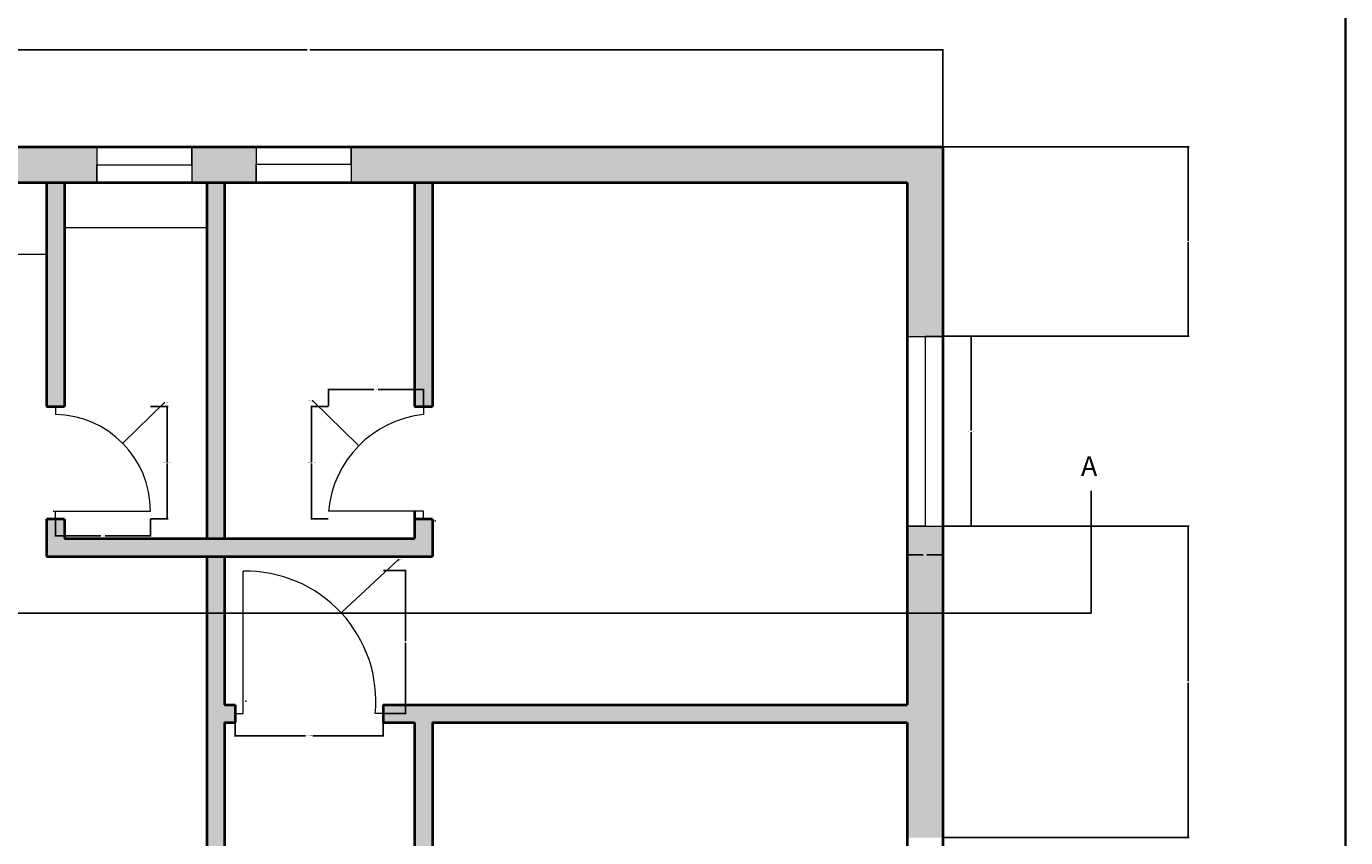
# Model space of a CAD drawing. Units: inches. Extents: x 1441 to 2460, y 1648 to 2683.
# Tile 33 of 35: x 2127 to 2460, y 2124 to 2329. Entities that reach past the tile are written whole.
import ezdxf

# ---------------------------------------------------------------- set-up
doc = ezdxf.new("R2010")
doc.units = ezdxf.units.IN
for name, color, linetype, lineweight in [('A-ANNO-DIMS', 2, 'Continuous', 18), ('A-ANNO-SYMB', 5, 'Continuous', 25), ('A-ANNO-TTLB', 7, 'Continuous', 35), ('A-DOOR', 3, 'Continuous', 20), ('A-FLOR-CASE', 9, 'Continuous', 20), ('A-GLAZ', 4, 'Continuous', 18), ('A-WALL', 7, 'Continuous', 40)]:
    doc.layers.add(name, color=color, linetype=linetype, lineweight=lineweight)
doc.layers.add('A-WALL-PATT', color=251, linetype='Continuous', lineweight=13, true_color=0x636466)
doc.styles.get("Standard").update_dxf_attribs({"font": 'arial.ttf'})
doc.dimstyles.get("Standard").update_dxf_attribs({"dimtxt": 0.18, "dimasz": 0.18, "dimexe": 0.18, "dimexo": 0.0625, "dimgap": 0.09, "dimtad": 0, "dimtih": 1, "dimtoh": 1, "dimdec": 4, "dimzin": 0, "dimdsep": 46, "dimtxsty": 'Standard', "dimcen": 0.09, "dimadec": 0, "dimazin": 0, "dimtfac": 1, "dimtdec": 4, "dimtofl": 0, "dimtmove": 0, "dimatfit": 3, "dimfxl": 1, "dimtolj": 1, "dimtzin": 0, "dimarcsym": 0})

# ---------------------------------------------------------------- blocks, each defined once
blk = doc.blocks.new('DOOR-BED1-36')
for p, q in [((2, 0), (2, 36)), ((0, 0), (2, 0)), ((37.39, 0), (35.39, 0))]:
    blk.add_line(p, q)
blk.add_arc((2.69, 3.15), 32.85, 354.488, 91.1985)
blk = doc.blocks.new('DOOR-WC-NORTH-24')
for p, q in [((24, 28.42), (24, 26.42)), ((24, 2), (0, 2)), ((24, 0), (24, 2))]:
    blk.add_line(p, q)
blk.add_arc((26.92, -0.45), 27.04, 96.2058, 174.7965)
blk = doc.blocks.new('DOOR-STORE-24')
for p, q in [((0, 28.42), (0, 26.42)), ((0, 0), (0, 2)), ((0, 2), (24, 2))]:
    blk.add_line(p, q)
blk.add_arc((-0.43, 2), 24.43, 0, 88.9938)
blk = doc.blocks.new('WIN-48-SASH')
for p, q in [((9, 48), (4.5, 48)), ((4.5, 48), (4.5, 0)), ((4.5, 0), (0, 0))]:
    blk.add_line(p, q)
blk = doc.blocks.new('*D42')
at = {"layer": 'A-ANNO-DIMS', "color": 0, "lineweight": -2, "transparency": 16777216}
for p, q in [((2179.58, 2155.38), (2179.58, 2149.66)), ((2216.96, 2155.38), (2216.96, 2149.66)), ((2179.76, 2149.84), (2197.34, 2149.84)), ((2216.78, 2149.84), (2199.2, 2149.84))]:
    blk.add_line(p, q, dxfattribs=at)
at = {"layer": 'A-ANNO-DIMS', "color": 0, "transparency": 16777216}
for points in [[(2179.76, 2149.87), (2179.76, 2149.81), (2179.58, 2149.84)], [(2216.78, 2149.87), (2216.78, 2149.81), (2216.96, 2149.84)]]:
    blk.add_solid(points, dxfattribs=at)
at = {"layer": 'Defpoints', "color": 0, "transparency": 16777216}
for p in [(2179.58, 2155.45), (2216.96, 2155.45), (2216.96, 2149.84)]:
    blk.add_point(p, dxfattribs=at)
at = {"layer": 'A-ANNO-DIMS', "color": 0, "transparency": 16777216, "insert": (2198.27, 2149.84), "char_height": 0.18, "attachment_point": 5}
blk.add_mtext('\\A1;B1 DR 37 TYP.', dxfattribs=at)
blk = doc.blocks.new('*D43')
at = {"layer": 'A-ANNO-DIMS', "color": 0, "lineweight": -2, "transparency": 16777216}
for p, q in [((2217.03, 2191.64), (2222.75, 2191.64)), ((2222.57, 2191.46), (2222.57, 2173.73)), ((2222.57, 2155.63), (2222.57, 2173.36)), ((2217.03, 2155.45), (2222.75, 2155.45))]:
    blk.add_line(p, q, dxfattribs=at)
at = {"layer": 'A-ANNO-DIMS', "color": 0, "transparency": 16777216}
for points in [[(2222.54, 2191.46), (2222.6, 2191.46), (2222.57, 2191.64)], [(2222.54, 2155.63), (2222.6, 2155.63), (2222.57, 2155.45)]]:
    blk.add_solid(points, dxfattribs=at)
at = {"layer": 'Defpoints', "color": 0, "transparency": 16777216}
for p in [(2216.96, 2191.64), (2222.57, 2191.64), (2216.96, 2155.45)]:
    blk.add_point(p, dxfattribs=at)
at = {"layer": 'A-ANNO-DIMS', "color": 0, "transparency": 16777216, "insert": (2222.57, 2173.54), "char_height": 0.18, "attachment_point": 5}
blk.add_mtext('\\A1;36 TYP.', dxfattribs=at)
blk = doc.blocks.new('*D44')
at = {"layer": 'A-ANNO-DIMS', "color": 0, "lineweight": -2, "transparency": 16777216}
for p, q in [((2203.09, 2233.06), (2198.71, 2233.06)), ((2198.89, 2232.88), (2198.89, 2219.03)), ((2198.89, 2204.82), (2198.89, 2218.67)), ((2203.09, 2204.64), (2198.71, 2204.64))]:
    blk.add_line(p, q, dxfattribs=at)
at = {"layer": 'A-ANNO-DIMS', "color": 0, "transparency": 16777216}
for points in [[(2198.86, 2232.88), (2198.92, 2232.88), (2198.89, 2233.06)], [(2198.86, 2204.82), (2198.92, 2204.82), (2198.89, 2204.64)]]:
    blk.add_solid(points, dxfattribs=at)
at = {"layer": 'Defpoints', "color": 0, "transparency": 16777216}
for p in [(2198.89, 2233.06), (2203.15, 2233.06), (2203.15, 2204.64)]:
    blk.add_point(p, dxfattribs=at)
at = {"layer": 'A-ANNO-DIMS', "color": 0, "transparency": 16777216, "insert": (2198.89, 2218.85), "char_height": 0.18, "attachment_point": 5}
blk.add_mtext('\\A1;WC DOOR 28 TYP.', dxfattribs=at)
blk = doc.blocks.new('*D45')
at = {"layer": 'A-ANNO-DIMS', "color": 0, "lineweight": -2, "transparency": 16777216}
for p, q in [((2203.15, 2233.12), (2203.15, 2237.51)), ((2203.33, 2237.33), (2214.62, 2237.33)), ((2226.97, 2237.33), (2215.68, 2237.33)), ((2227.15, 2233.12), (2227.15, 2237.51))]:
    blk.add_line(p, q, dxfattribs=at)
at = {"layer": 'A-ANNO-DIMS', "color": 0, "transparency": 16777216}
for points in [[(2203.33, 2237.36), (2203.33, 2237.3), (2203.15, 2237.33)], [(2226.97, 2237.36), (2226.97, 2237.3), (2227.15, 2237.33)]]:
    blk.add_solid(points, dxfattribs=at)
at = {"layer": 'Defpoints', "color": 0, "transparency": 16777216}
for p in [(2227.15, 2237.33), (2203.15, 2233.06), (2227.15, 2233.06)]:
    blk.add_point(p, dxfattribs=at)
at = {"layer": 'A-ANNO-DIMS', "color": 0, "transparency": 16777216, "insert": (2215.15, 2237.33), "char_height": 0.18, "attachment_point": 5}
blk.add_mtext('\\A1;24 TYP.', dxfattribs=at)
blk = doc.blocks.new('*D46')
at = {"layer": 'A-ANNO-DIMS', "color": 0, "lineweight": -2, "transparency": 16777216}
for p, q in [((2158.21, 2233.06), (2162.6, 2233.06)), ((2162.42, 2232.88), (2162.42, 2219.03)), ((2162.42, 2204.82), (2162.42, 2218.67)), ((2158.21, 2204.64), (2162.6, 2204.64))]:
    blk.add_line(p, q, dxfattribs=at)
at = {"layer": 'A-ANNO-DIMS', "color": 0, "transparency": 16777216}
for points in [[(2162.39, 2232.88), (2162.45, 2232.88), (2162.42, 2233.06)], [(2162.39, 2204.82), (2162.45, 2204.82), (2162.42, 2204.64)]]:
    blk.add_solid(points, dxfattribs=at)
at = {"layer": 'Defpoints', "color": 0, "transparency": 16777216}
for p in [(2158.15, 2233.06), (2162.42, 2233.06), (2158.15, 2204.64)]:
    blk.add_point(p, dxfattribs=at)
at = {"layer": 'A-ANNO-DIMS', "color": 0, "transparency": 16777216, "insert": (2162.42, 2218.85), "char_height": 0.18, "attachment_point": 5}
blk.add_mtext('\\A1;STORE DOOR 28 TYP.', dxfattribs=at)
blk = doc.blocks.new('*D47')
at = {"layer": 'A-ANNO-DIMS', "color": 0, "lineweight": -2, "transparency": 16777216}
for p, q in [((2134.15, 2204.57), (2134.15, 2200.19)), ((2158.15, 2204.57), (2158.15, 2200.19)), ((2134.33, 2200.37), (2145.62, 2200.37)), ((2157.97, 2200.37), (2146.68, 2200.37))]:
    blk.add_line(p, q, dxfattribs=at)
at = {"layer": 'A-ANNO-DIMS', "color": 0, "transparency": 16777216}
for points in [[(2134.33, 2200.4), (2134.33, 2200.34), (2134.15, 2200.37)], [(2157.97, 2200.4), (2157.97, 2200.34), (2158.15, 2200.37)]]:
    blk.add_solid(points, dxfattribs=at)
at = {"layer": 'Defpoints', "color": 0, "transparency": 16777216}
for p in [(2134.15, 2204.64), (2158.15, 2204.64), (2158.15, 2200.37)]:
    blk.add_point(p, dxfattribs=at)
at = {"layer": 'A-ANNO-DIMS', "color": 0, "transparency": 16777216, "insert": (2146.15, 2200.37), "char_height": 0.18, "attachment_point": 5}
blk.add_mtext('\\A1;24 TYP.', dxfattribs=at)
blk = doc.blocks.new('*D58')
at = {"layer": 'A-ANNO-DIMS', "color": 0, "lineweight": -2, "transparency": 16777216}
for p, q in [((2358.46, 2250.81), (2365.78, 2250.81)), ((2365.6, 2250.63), (2365.6, 2226.99)), ((2365.6, 2202.99), (2365.6, 2226.62)), ((2358.46, 2202.81), (2365.78, 2202.81))]:
    blk.add_line(p, q, dxfattribs=at)
at = {"layer": 'A-ANNO-DIMS', "color": 0, "transparency": 16777216}
for points in [[(2365.57, 2250.63), (2365.63, 2250.63), (2365.6, 2250.81)], [(2365.57, 2202.99), (2365.63, 2202.99), (2365.6, 2202.81)]]:
    blk.add_solid(points, dxfattribs=at)
at = {"layer": 'Defpoints', "color": 0, "transparency": 16777216}
for p in [(2358.4, 2250.81), (2365.6, 2250.81), (2358.4, 2202.81)]:
    blk.add_point(p, dxfattribs=at)
at = {"layer": 'A-ANNO-DIMS', "color": 0, "transparency": 16777216, "insert": (2365.6, 2226.81), "char_height": 0.18, "attachment_point": 5}
blk.add_mtext('\\A1;SASH 48 TYP.', dxfattribs=at)
blk = doc.blocks.new('*D59')
at = {"layer": 'A-ANNO-DIMS', "color": 0, "lineweight": -2, "transparency": 16777216}
for p, q in [((2349.4, 2202.74), (2349.4, 2195.43)), ((2358.4, 2202.74), (2358.4, 2195.43)), ((2349.58, 2195.61), (2353.44, 2195.61)), ((2358.22, 2195.61), (2354.36, 2195.61))]:
    blk.add_line(p, q, dxfattribs=at)
at = {"layer": 'A-ANNO-DIMS', "color": 0, "transparency": 16777216}
for points in [[(2349.58, 2195.64), (2349.58, 2195.58), (2349.4, 2195.61)], [(2358.22, 2195.64), (2358.22, 2195.58), (2358.4, 2195.61)]]:
    blk.add_solid(points, dxfattribs=at)
at = {"layer": 'Defpoints', "color": 0, "transparency": 16777216}
for p in [(2349.4, 2202.81), (2358.4, 2202.81), (2358.4, 2195.61)]:
    blk.add_point(p, dxfattribs=at)
at = {"layer": 'A-ANNO-DIMS', "color": 0, "transparency": 16777216, "insert": (2353.9, 2195.61), "char_height": 0.18, "attachment_point": 5}
blk.add_mtext('\\A1;9 TYP.', dxfattribs=at)
blk = doc.blocks.new('*D80')
at = {"layer": 'A-ANNO-DIMS', "color": 0, "lineweight": -2, "transparency": 16777216}
for p, q in [((2037.9, 2298.76), (2037.9, 2323.43)), ((2038.08, 2323.25), (2197.76, 2323.25)), ((2358.22, 2323.25), (2198.55, 2323.25)), ((2358.4, 2298.76), (2358.4, 2323.43))]:
    blk.add_line(p, q, dxfattribs=at)
at = {"layer": 'A-ANNO-DIMS', "color": 0, "transparency": 16777216}
for points in [[(2038.08, 2323.28), (2038.08, 2323.22), (2037.9, 2323.25)], [(2358.22, 2323.28), (2358.22, 2323.22), (2358.4, 2323.25)]]:
    blk.add_solid(points, dxfattribs=at)
at = {"layer": 'Defpoints', "color": 0, "transparency": 16777216}
for p in [(2358.4, 2323.25), (2037.9, 2298.7), (2358.4, 2298.7)]:
    blk.add_point(p, dxfattribs=at)
at = {"layer": 'A-ANNO-DIMS', "color": 0, "transparency": 16777216, "insert": (2198.15, 2323.25), "char_height": 0.18, "attachment_point": 5}
blk.add_mtext('\\A1;320.5', dxfattribs=at)
blk = doc.blocks.new('*D81')
at = {"layer": 'A-ANNO-DIMS', "color": 0, "lineweight": -2, "transparency": 16777216}
for p, q in [((2037.84, 2298.7), (1976.42, 2298.7)), ((1976.6, 2298.52), (1976.6, 2055.94)), ((1976.6, 1813), (1976.6, 2055.57)), ((2154.24, 1812.82), (1976.42, 1812.82))]:
    blk.add_line(p, q, dxfattribs=at)
at = {"layer": 'A-ANNO-DIMS', "color": 0, "transparency": 16777216}
for points in [[(1976.57, 2298.52), (1976.63, 2298.52), (1976.6, 2298.7)], [(1976.57, 1813), (1976.63, 1813), (1976.6, 1812.82)]]:
    blk.add_solid(points, dxfattribs=at)
at = {"layer": 'Defpoints', "color": 0, "transparency": 16777216}
for p in [(1976.6, 2298.7), (2037.9, 2298.7), (2154.3, 1812.82)]:
    blk.add_point(p, dxfattribs=at)
at = {"layer": 'A-ANNO-DIMS', "color": 0, "transparency": 16777216, "insert": (1976.6, 2055.76), "char_height": 0.18, "attachment_point": 5}
blk.add_mtext('\\A1;485.9', dxfattribs=at)
blk = doc.blocks.new('*D88')
at = {"layer": 'A-ANNO-DIMS', "color": 0, "lineweight": -2, "transparency": 16777216}
for p, q in [((2358.46, 2202.81), (2420.62, 2202.81)), ((2420.44, 2202.63), (2420.44, 2163.64)), ((2420.44, 2124.29), (2420.44, 2163.27)), ((2358.46, 2124.11), (2420.62, 2124.11))]:
    blk.add_line(p, q, dxfattribs=at)
at = {"layer": 'A-ANNO-DIMS', "color": 0, "transparency": 16777216}
for points in [[(2420.41, 2202.63), (2420.47, 2202.63), (2420.44, 2202.81)], [(2420.41, 2124.29), (2420.47, 2124.29), (2420.44, 2124.11)]]:
    blk.add_solid(points, dxfattribs=at)
at = {"layer": 'Defpoints', "color": 0, "transparency": 16777216}
for p in [(2358.4, 2202.81), (2420.44, 2202.81), (2358.4, 2124.11)]:
    blk.add_point(p, dxfattribs=at)
at = {"layer": 'A-ANNO-DIMS', "color": 0, "transparency": 16777216, "insert": (2420.44, 2163.46), "char_height": 0.18, "attachment_point": 5}
blk.add_mtext('\\A1;78.7', dxfattribs=at)
blk = doc.blocks.new('*D89')
at = {"layer": 'A-ANNO-DIMS', "color": 0, "lineweight": -2, "transparency": 16777216}
for p, q in [((2358.46, 2298.7), (2420.62, 2298.7)), ((2420.44, 2298.52), (2420.44, 2274.93)), ((2420.44, 2250.99), (2420.44, 2274.57)), ((2358.46, 2250.81), (2420.62, 2250.81))]:
    blk.add_line(p, q, dxfattribs=at)
at = {"layer": 'A-ANNO-DIMS', "color": 0, "transparency": 16777216}
for points in [[(2420.41, 2298.52), (2420.47, 2298.52), (2420.44, 2298.7)], [(2420.41, 2250.99), (2420.47, 2250.99), (2420.44, 2250.81)]]:
    blk.add_solid(points, dxfattribs=at)
at = {"layer": 'Defpoints', "color": 0, "transparency": 16777216}
for p in [(2358.4, 2298.7), (2420.44, 2298.7), (2358.4, 2250.81)]:
    blk.add_point(p, dxfattribs=at)
at = {"layer": 'A-ANNO-DIMS', "color": 0, "transparency": 16777216, "insert": (2420.44, 2274.75), "char_height": 0.18, "attachment_point": 5}
blk.add_mtext('\\A1;47.89', dxfattribs=at)
blk = doc.blocks.new('*D130')
at = {"layer": 'A-ANNO-DIMS', "color": 0, "lineweight": -2, "transparency": 16777216}
for p, q in [((2220.8, 2194.34), (2206.48, 2181.06)), ((2220.98, 2194.34), (2220.8, 2194.34)), ((2182.17, 2158.6), (2182.35, 2158.6)), ((2182.26, 2158.51), (2182.26, 2158.69))]:
    blk.add_line(p, q, dxfattribs=at)
at = {"layer": 'A-ANNO-DIMS', "color": 0, "transparency": 16777216}
blk.add_solid([(2206.46, 2181.08), (2206.5, 2181.04), (2206.35, 2180.94)], dxfattribs=at)
at = {"layer": 'Defpoints', "color": 0, "transparency": 16777216}
for p in [(2206.35, 2180.94), (2182.26, 2158.6)]:
    blk.add_point(p, dxfattribs=at)
at = {"layer": 'A-ANNO-DIMS', "color": 0, "transparency": 16777216, "insert": (2221.46, 2194.34), "char_height": 0.18, "attachment_point": 5}
blk.add_mtext('\\A1;R32.85', dxfattribs=at)
blk = doc.blocks.new('*D133')
at = {"layer": 'A-ANNO-DIMS', "color": 0, "lineweight": -2, "transparency": 16777216}
for p, q in [((2199.04, 2234.5), (2199.22, 2234.5)), ((2199.22, 2234.5), (2210.66, 2223.26)), ((2229.99, 2204.19), (2230.17, 2204.19)), ((2230.08, 2204.1), (2230.08, 2204.28))]:
    blk.add_line(p, q, dxfattribs=at)
at = {"layer": 'A-ANNO-DIMS', "color": 0, "transparency": 16777216}
blk.add_solid([(2210.68, 2223.28), (2210.64, 2223.24), (2210.79, 2223.13)], dxfattribs=at)
at = {"layer": 'Defpoints', "color": 0, "transparency": 16777216}
for p in [(2210.79, 2223.13), (2230.08, 2204.19)]:
    blk.add_point(p, dxfattribs=at)
at = {"layer": 'A-ANNO-DIMS', "color": 0, "transparency": 16777216, "insert": (2198.49, 2234.5), "char_height": 0.18, "attachment_point": 5}
blk.add_mtext('\\A1;R27.036', dxfattribs=at)
blk = doc.blocks.new('*D134')
at = {"layer": 'A-ANNO-DIMS', "color": 0, "lineweight": -2, "transparency": 16777216}
for p, q in [((2161.6, 2234.03), (2151.28, 2223.89)), ((2161.78, 2234.03), (2161.6, 2234.03)), ((2133.63, 2206.64), (2133.81, 2206.64)), ((2133.72, 2206.55), (2133.72, 2206.73))]:
    blk.add_line(p, q, dxfattribs=at)
at = {"layer": 'A-ANNO-DIMS', "color": 0, "transparency": 16777216}
blk.add_solid([(2151.25, 2223.91), (2151.3, 2223.86), (2151.15, 2223.76)], dxfattribs=at)
at = {"layer": 'Defpoints', "color": 0, "transparency": 16777216}
for p in [(2151.15, 2223.76), (2133.72, 2206.64)]:
    blk.add_point(p, dxfattribs=at)
at = {"layer": 'A-ANNO-DIMS', "color": 0, "transparency": 16777216, "insert": (2162.26, 2234.03), "char_height": 0.18, "attachment_point": 5}
blk.add_mtext('\\A1;R24.43', dxfattribs=at)

msp = doc.modelspace()

# ---------------------------------------------------------------- hatches: boundary and pattern name
at = {"layer": 'A-WALL-PATT'}
h = msp.add_hatch(color=256, dxfattribs=at)
h.dxf.hatch_style = 1
h.paths.add_polyline_path([(2096.524, 2298.6952), (2037.9015, 2298.6952), (2037.9015, 2246.9605), (2046.9015, 2246.9605), (2046.9015, 2289.6952), (2096.524, 2289.6952), (2096.524, 2294.1952)])
h.paths.add_polyline_path([(2144.5933, 2298.6952), (2120.524, 2298.6952), (2120.524, 2289.6952), (2144.5933, 2289.6952), (2144.5933, 2294.1952)])
h.paths.add_polyline_path([(2136.4015, 2289.6952), (2131.9015, 2289.6952), (2131.9015, 2233.0622), (2136.4015, 2233.0622)])
h.paths.add_polyline_path([(2184.8877, 2294.3362), (2184.8877, 2295.2788), (2184.8877, 2298.6952), (2168.5933, 2298.6952), (2168.5933, 2289.6952), (2184.8877, 2289.6952)])
h.paths.add_polyline_path([(2176.9015, 2289.6952), (2172.4015, 2289.6952), (2172.4015, 2199.6952), (2176.9015, 2199.6952)])
h.paths.add_polyline_path([(2229.4015, 2204.637), (2224.9015, 2204.637), (2224.9015, 2199.6952), (2136.4015, 2199.6952), (2136.4015, 2204.637), (2131.9015, 2204.637), (2131.9015, 2195.1952), (2229.4015, 2195.1952)])
h.paths.add_polyline_path([(2229.4015, 2289.6952), (2224.9015, 2289.6952), (2224.9015, 2233.0622), (2229.4015, 2233.0622)])
h.paths.add_polyline_path([(2358.4015, 2298.6952), (2208.8877, 2298.6952), (2208.8877, 2289.6952), (2349.4015, 2289.6952), (2349.4015, 2250.8051), (2358.4015, 2250.8051)])
h.paths.add_polyline_path([(2358.4015, 2202.8051), (2349.4015, 2202.8051), (2349.4015, 2157.6952), (2216.9636, 2157.6952), (2216.9636, 2153.1952), (2224.9015, 2153.1952), (2224.9015, 2058.005), (2229.4015, 2058.005), (2229.4015, 2153.1952), (2349.4015, 2153.1952), (2349.4015, 2124.108), (2358.4015, 2124.108)])
h.paths.add_polyline_path([(2358.4015, 1984.8305), (2349.4015, 1984.8305), (2349.4015, 1834.1952), (2358.4015, 1834.1952)])
h.paths.add_polyline_path([(2358.4015, 2076.108), (2349.4015, 2076.108), (2349.4015, 2008.8305), (2358.4015, 2008.8305)])
h.paths.add_polyline_path([(2349.4015, 2027.1952), (2269.9015, 2027.1952), (2269.9015, 2000.9452), (2274.4015, 2000.9452), (2274.4015, 2022.6952), (2349.4015, 2022.6952)])
h.paths.add_polyline_path([(2269.9015, 2027.1952), (2229.4015, 2027.1952), (2229.4015, 2030.7912), (2224.9015, 2030.7912), (2224.9015, 2022.6952), (2269.9015, 2022.6952)])
h.paths.add_polyline_path([(2349.4015, 1974.6952), (2274.4015, 1974.6952), (2274.4015, 1978.7973), (2269.9015, 1978.7973), (2269.9015, 1974.6952), (2263.8979, 1974.6952), (2263.8979, 1970.1952), (2269.9015, 1970.1952), (2274.4015, 1970.1952), (2349.4015, 1970.1952)])
h.paths.add_polyline_path([(2229.4015, 1974.6952), (2224.9015, 1974.6952), (2224.9015, 1925.6952), (2220.8772, 1925.6952), (2220.8772, 1921.1952), (2229.4015, 1921.1952)])
h.paths.add_polyline_path([(2229.4015, 1921.1952), (2224.9015, 1921.1952), (2224.9015, 1843.1952), (2229.4015, 1843.1952)])
h.paths.add_polyline_path([(2268.1291, 1838.6952), (2268.1291, 1843.1952), (2229.4015, 1843.1952), (2220.91, 1843.1952), (2220.91, 1834.1952), (2227.1771, 1834.1952), (2268.1291, 1834.1952)])
h.paths.add_polyline_path([(2349.4015, 1843.1952), (2328.1291, 1843.1952), (2328.1291, 1834.1952), (2349.4015, 1834.1952)])
h.paths.add_polyline_path([(2046.9015, 1857.7914), (2037.9015, 1857.7914), (2037.9015, 1834.1952), (2164.019, 1834.1952), (2164.019, 1838.6952), (2164.019, 1843.1952), (2046.9015, 1843.1952)])
h.paths.add_polyline_path([(2046.9015, 1959.2399), (2042.4015, 1959.2399), (2037.9015, 1959.2399), (2037.9015, 1905.7914), (2046.9015, 1905.7914), (2046.9015, 1921.1952), (2172.4015, 1921.1952), (2176.9015, 1921.1952), (2184.1657, 1921.1952), (2184.1657, 1925.6952), (2176.9015, 1925.6952), (2172.4015, 1925.6952), (2046.9015, 1925.6952)])
h.paths.add_polyline_path([(2046.9015, 2106.6907), (2037.9015, 2106.6907), (2037.9015, 2019.2399), (2046.9015, 2019.2399)])
h.paths.add_polyline_path([(2176.9015, 2051.6952), (2172.4015, 2051.6952), (2172.4015, 2048.6952), (2172.4015, 1925.6952), (2176.9015, 1925.6952)])
h.paths.add_polyline_path([(2172.4015, 2051.6952), (2145.4015, 2051.6952), (2145.4015, 2048.6952), (2172.4015, 2048.6952)])
h.paths.add_polyline_path([(2172.4015, 2102.6952), (2145.4015, 2102.6952), (2145.4015, 2099.6952), (2154.4015, 2099.6952), (2172.4015, 2099.6952)])
h.paths.add_polyline_path([(2176.9015, 2153.1952), (2179.5767, 2153.1952), (2179.5767, 2157.6952), (2176.9015, 2157.6952), (2176.9015, 2195.1952), (2172.4015, 2195.1952), (2172.4015, 2099.6952), (2176.9015, 2099.6952)])
h.paths.add_polyline_path([(2046.9015, 2198.9605), (2037.9015, 2198.9605), (2037.9015, 2166.6907), (2046.9015, 2166.6907)])

# ---------------------------------------------------------------- linework, layer by layer
at = {"layer": 'A-ANNO-SYMB'}
for p, q in [((2395.889, 2180.8746), (2395.889, 2211.7201)), ((2001.1539, 2180.8746), (2395.889, 2180.8746))]:
    msp.add_line(p, q, dxfattribs=at)
at = {"layer": 'A-ANNO-TTLB'}
msp.add_lwpolyline([(1440.5107, 2682.6413), (2460.193, 2682.6413), (2460.193, 1648.08), (1440.5107, 1648.08)], close=True, dxfattribs=at)
at = {"layer": 'A-FLOR-CASE'}
for p, q in [((2136.4015, 2278.307), (2172.4015, 2278.307)), ((2069.5886, 2271.5733), (2131.9015, 2271.5733))]:
    msp.add_line(p, q, dxfattribs=at)
at = {"layer": 'A-GLAZ'}
for p, q in [((2144.5933, 2298.6952), (2144.5933, 2289.6952)), ((2168.5933, 2294.1952), (2168.5933, 2298.6952)), ((2168.5933, 2298.6952), (2168.5933, 2289.6952)), ((2184.8877, 2298.6952), (2184.8877, 2295.2788)), ((2208.8877, 2294.3362), (2208.8877, 2298.6952)), ((2208.8877, 2298.6952), (2208.8877, 2289.6952)), ((2144.5933, 2289.6952), (2144.5933, 2294.1952)), ((2144.5933, 2294.1952), (2168.5933, 2294.1952)), ((2184.8877, 2295.2788), (2184.8877, 2289.6952)), ((2184.8877, 2289.6952), (2184.8877, 2294.3362)), ((2184.8877, 2294.3362), (2208.8877, 2294.3362)), ((2349.4015, 2250.8051), (2358.4015, 2250.8051)), ((2349.4015, 2202.8051), (2358.4015, 2202.8051))]:
    msp.add_line(p, q, dxfattribs=at)
at = {"layer": 'A-WALL'}
for p, q in [((2037.9015, 2298.6952), (2358.4015, 2298.6952)), ((2358.4015, 2298.6952), (2358.4015, 1834.1952)), ((2046.9015, 2289.6952), (2349.4015, 2289.6952)), ((2131.9015, 2289.6952), (2131.9015, 2233.0622)), ((2136.4015, 2289.6952), (2136.4015, 2233.0622)), ((2172.4015, 2289.6952), (2172.4015, 2199.6952)), ((2176.9015, 2289.6952), (2176.9015, 2199.6952)), ((2224.9015, 2289.6952), (2224.9015, 2233.0622)), ((2229.4015, 2289.6952), (2229.4015, 2233.0622)), ((2349.4015, 2289.6952), (2349.4015, 2157.6952)), ((2131.9015, 2233.0622), (2136.4015, 2233.0622)), ((2224.9015, 2233.0622), (2229.4015, 2233.0622)), ((2131.9015, 2204.637), (2131.9015, 2195.1952)), ((2136.4015, 2204.637), (2131.9015, 2204.637)), ((2136.4015, 2204.637), (2136.4015, 2199.6952)), ((2224.9015, 2206.637), (2224.9015, 2199.6952)), ((2229.4015, 2204.637), (2224.9015, 2204.637)), ((2229.4015, 2204.637), (2229.4015, 2195.1952)), ((2136.4015, 2199.6952), (2224.9015, 2199.6952)), ((2131.9015, 2195.1952), (2229.4015, 2195.1952)), ((2172.4015, 2195.1952), (2172.4015, 2099.6952)), ((2176.9015, 2195.1952), (2176.9015, 2157.6952)), ((2349.4015, 2195.1952), (2349.4015, 2157.6952)), ((2176.9015, 2157.6952), (2179.5767, 2157.6952)), ((2179.5767, 2157.6952), (2179.5767, 2153.1952)), ((2216.9636, 2157.6952), (2349.4015, 2157.6952)), ((2216.9636, 2157.6952), (2216.9636, 2153.1952)), ((2176.9015, 2153.1952), (2176.9015, 2099.6952)), ((2176.9015, 2153.1952), (2179.5767, 2153.1952)), ((2216.9636, 2153.1952), (2224.9015, 2153.1952)), ((2224.9015, 2153.1952), (2224.9015, 2058.005)), ((2229.4015, 2153.1952), (2229.4015, 2058.005)), ((2229.4015, 2153.1952), (2349.4015, 2153.1952)), ((2349.4015, 2153.1952), (2349.4015, 1834.1952))]:
    msp.add_line(p, q, dxfattribs=at)

# ---------------------------------------------------------------- block references
at = {"layer": 'A-DOOR'}
for name, p in [('DOOR-STORE-24', (2134.1556, 2204.64)), ('DOOR-WC-NORTH-24', (2203.1556, 2204.64)), ('DOOR-BED1-36', (2179.5756, 2155.45))]:
    msp.add_blockref(name, p, dxfattribs=at)
at = {"layer": 'A-GLAZ'}
msp.add_blockref('WIN-48-SASH', (2349.4056, 2202.8045), dxfattribs=at)

# ---------------------------------------------------------------- texts
at = {"layer": 'A-ANNO-SYMB', "insert": (2393.303, 2220.4981), "char_height": 5, "attachment_point": 1}
msp.add_mtext_dynamic_manual_height_columns('A', width=32.073624, gutter_width=12.5, heights=[0], dxfattribs=at)

# ---------------------------------------------------------------- dimensions: what is measured, and where the dimension line sits
at = {"layer": 'A-ANNO-DIMS'}
dim = msp.add_linear_dim(base=(2358.4015, 2323.2452), p1=(2037.9015, 2298.6952), p2=(2358.4015, 2298.6952), dimstyle='Standard', override={"dimdec": 1, "dimlfac": 1, "dimrnd": 0, "dimzin": 0, "dimdsep": 46, "dimlunit": 2}, dxfattribs=at)
dim.commit()
dim.dimension.update_dxf_attribs({"geometry": '*D80', "text_midpoint": (2198.1515, 2323.2452)})
for base, p1, p2, override, picture, middle in [((1976.6039, 2298.6952), (2154.3041, 1812.8171), (2037.9015, 2298.6952), {"dimdec": 1, "dimlfac": 1, "dimrnd": 0, "dimzin": 0, "dimdsep": 46, "dimlunit": 2}, '*D81', (1976.6039, 2055.7561)), ((2420.439, 2298.6952), (2358.4015, 2250.8051), (2358.4015, 2298.6952), {"dimdec": 2, "dimlfac": 1, "dimrnd": 0, "dimzin": 0, "dimdsep": 46, "dimlunit": 2}, '*D89', (2420.439, 2274.7501)), ((2420.439, 2202.8051), (2358.4015, 2124.108), (2358.4015, 2202.8051), {"dimdec": 1, "dimlfac": 1, "dimrnd": 0, "dimzin": 0, "dimdsep": 46, "dimlunit": 2}, '*D88', (2420.439, 2163.4565))]:
    dim = msp.add_linear_dim(base=base, p1=p1, p2=p2, angle=90, dimstyle='Standard', override=override, dxfattribs=at)
    dim.commit()
    dim.dimension.update_dxf_attribs({"geometry": picture, "text_midpoint": middle})
for base, p1, p2, text, picture, middle in [((2365.6015, 2250.8051), (2358.4015, 2202.8051), (2358.4015, 2250.8051), 'SASH <> TYP.', '*D58', (2365.6015, 2226.8051)), ((2162.4153, 2233.0622), (2158.1515, 2204.637), (2158.1515, 2233.0622), 'STORE DOOR <> TYP.', '*D46', (2162.4153, 2218.8496)), ((2198.8877, 2233.0622), (2203.1515, 2204.637), (2203.1515, 2233.0622), 'WC DOOR <> TYP.', '*D44', (2198.8877, 2218.8496)), ((2222.5716, 2191.6414), (2216.9636, 2155.4452), (2216.9636, 2191.6414), '<> TYP.', '*D43', (2222.5716, 2173.5433))]:
    dim = msp.add_linear_dim(base=base, p1=p1, p2=p2, angle=90, text=text, dimstyle='Standard', override={"dimdec": 0, "dimlfac": 1, "dimrnd": 0, "dimzin": 0, "dimdsep": 46, "dimlunit": 2}, dxfattribs=at)
    dim.commit()
    dim.dimension.update_dxf_attribs({"geometry": picture, "text_midpoint": middle})
for base, p1, p2, text, picture, middle in [((2227.1531, 2237.326), (2203.1515, 2233.0622), (2227.1531, 2233.0622), '<> TYP.', '*D45', (2215.1523, 2237.326)), ((2158.1515, 2200.3732), (2134.1515, 2204.637), (2158.1515, 2204.637), '<> TYP.', '*D47', (2146.1515, 2200.3732)), ((2358.4015, 2195.6051), (2349.4015, 2202.8051), (2358.4015, 2202.8051), '<> TYP.', '*D59', (2353.9015, 2195.6051)), ((2216.9636, 2149.8372), (2179.5767, 2155.4452), (2216.9636, 2155.4452), 'B1 DR <> TYP.', '*D42', (2198.2702, 2149.8372))]:
    dim = msp.add_linear_dim(base=base, p1=p1, p2=p2, text=text, dimstyle='Standard', override={"dimdec": 0, "dimlfac": 1, "dimrnd": 0, "dimzin": 0, "dimdsep": 46, "dimlunit": 2}, dxfattribs=at)
    dim.commit()
    dim.dimension.update_dxf_attribs({"geometry": picture, "text_midpoint": middle})
for center, mpoint, override, picture, middle in [((2133.7225, 2206.637), (2151.147, 2223.759), {"dimdec": 2, "dimlfac": 1, "dimrnd": 0, "dimzin": 0, "dimdsep": 46, "dimlunit": 2}, '*D134', (2162.2615, 2234.0322)), ((2230.0757, 2204.185), (2210.792, 2223.134), {"dimdec": 3, "dimlfac": 1, "dimrnd": 0, "dimzin": 0, "dimdsep": 46, "dimlunit": 2}, '*D133', (2198.4921, 2234.5034)), ((2182.2639, 2158.6007), (2206.351, 2180.94), {"dimdec": 2, "dimlfac": 1, "dimrnd": 0, "dimzin": 0, "dimdsep": 46, "dimlunit": 2}, '*D130', (2221.4638, 2194.3435))]:
    dim = msp.add_radius_dim(center=center, mpoint=mpoint, dimstyle='Standard', override=override, dxfattribs=at)
    dim.commit()
    dim.dimension.update_dxf_attribs({"geometry": picture, "text_midpoint": middle, "dimtype": 164})

doc.saveas('drawing.dxf')
